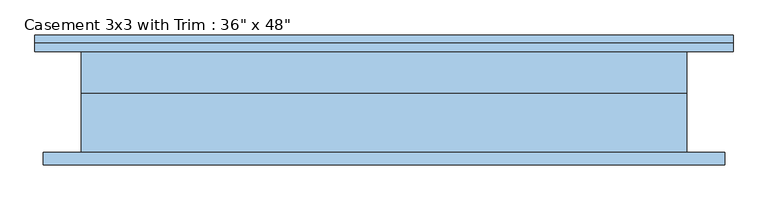
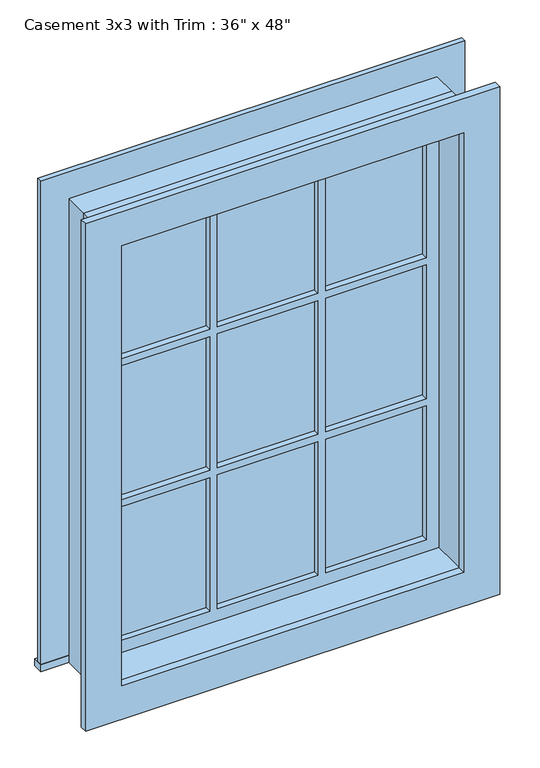
"""IFC4 building model written with IfcOpenShell, lengths in millimetres: window geometry."""

from ifc_helpers import new_model, si_unit, frame, origin, place, context, project, spatial, polyline, outline, extrude, source, transform, mapped, element, save


def window_5c190c7e(model_context):
    return source(origin(), model_context, "Body", "SweptSolid", [
        extrude(outline(polyline([(-527.05, 101.6), (527.05, 101.6), (527.05, 76.2), (-527.05, 76.2), (-527.05, 101.6)])), frame((0.0, 0.0, 914.4), z_axis=(0.0, 0.0, 1.0), x_axis=(1.0, 0.0, 0.0)), (0.0, 0.0, 1.0), 19.05),
        extrude(outline(polyline([(2114.55, -438.15), (2114.55, 438.15), (933.45, 438.15), (933.45, 527.05), (2203.45, 527.05), (2203.45, -527.05), (933.45, -527.05), (933.45, -438.15), (2114.55, -438.15)])), frame((0.0, 76.2, 0.0), z_axis=(0.0, 1.0, 0.0), x_axis=(0.0, 0.0, 1.0)), (0.0, 0.0, 1.0), 12.7),
        extrude(outline(polyline([(143.9333333, 41.275), (393.7, 41.275), (393.7, 28.575), (143.9333333, 28.575), (143.9333333, 41.275)])), frame((0.0, 0.0, 1718.7333333), z_axis=(0.0, 0.0, 1.0), x_axis=(1.0, 0.0, 0.0)), (0.0, 0.0, 1.0), 351.3666667),
        extrude(outline(polyline([(-124.8833333, 41.275), (124.8833333, 41.275), (124.8833333, 28.575), (-124.8833333, 28.575), (-124.8833333, 41.275)])), frame((0.0, 0.0, 1718.7333333), z_axis=(0.0, 0.0, 1.0), x_axis=(1.0, 0.0, 0.0)), (0.0, 0.0, 1.0), 351.3666667),
        extrude(outline(polyline([(-393.7, 41.275), (-143.9333333, 41.275), (-143.9333333, 28.575), (-393.7, 28.575), (-393.7, 41.275)])), frame((0.0, 0.0, 1718.7333333), z_axis=(0.0, 0.0, 1.0), x_axis=(1.0, 0.0, 0.0)), (0.0, 0.0, 1.0), 351.3666667),
        extrude(outline(polyline([(-393.7, 41.275), (-143.9333333, 41.275), (-143.9333333, 28.575), (-393.7, 28.575), (-393.7, 41.275)])), frame((0.0, 0.0, 1348.3166667), z_axis=(0.0, 0.0, 1.0), x_axis=(1.0, 0.0, 0.0)), (0.0, 0.0, 1.0), 351.3666667),
        extrude(outline(polyline([(-124.8833333, 41.275), (124.8833333, 41.275), (124.8833333, 28.575), (-124.8833333, 28.575), (-124.8833333, 41.275)])), frame((0.0, 0.0, 1348.3166667), z_axis=(0.0, 0.0, 1.0), x_axis=(1.0, 0.0, 0.0)), (0.0, 0.0, 1.0), 351.3666667),
        extrude(outline(polyline([(143.9333333, 41.275), (393.7, 41.275), (393.7, 28.575), (143.9333333, 28.575), (143.9333333, 41.275)])), frame((0.0, 0.0, 1348.3166667), z_axis=(0.0, 0.0, 1.0), x_axis=(1.0, 0.0, 0.0)), (0.0, 0.0, 1.0), 351.3666667),
        extrude(outline(polyline([(143.9333333, 41.275), (393.7, 41.275), (393.7, 28.575), (143.9333333, 28.575), (143.9333333, 41.275)])), frame((0.0, 0.0, 977.9), z_axis=(0.0, 0.0, 1.0), x_axis=(1.0, 0.0, 0.0)), (0.0, 0.0, 1.0), 351.3666667),
        extrude(outline(polyline([(-124.8833333, 41.275), (124.8833333, 41.275), (124.8833333, 28.575), (-124.8833333, 28.575), (-124.8833333, 41.275)])), frame((0.0, 0.0, 977.9), z_axis=(0.0, 0.0, 1.0), x_axis=(1.0, 0.0, 0.0)), (0.0, 0.0, 1.0), 351.3666667),
        extrude(outline(polyline([(-393.7, 41.275), (-143.9333333, 41.275), (-143.9333333, 28.575), (-393.7, 28.575), (-393.7, 41.275)])), frame((0.0, 0.0, 977.9), z_axis=(0.0, 0.0, 1.0), x_axis=(1.0, 0.0, 0.0)), (0.0, 0.0, 1.0), 351.3666667),
        extrude(outline(polyline([(2190.75, 514.35), (2190.75, -514.35), (857.25, -514.35), (857.25, 514.35), (2190.75, 514.35)]), holes=[polyline([(2101.85, 425.45), (946.15, 425.45), (946.15, -425.45), (2101.85, -425.45), (2101.85, 425.45)])]), frame((0.0, -95.25, 0.0), z_axis=(0.0, 1.0, 0.0), x_axis=(0.0, 0.0, 1.0)), (0.0, 0.0, 1.0), 19.05),
        extrude(outline(polyline([(2114.55, -438.15), (933.45, -438.15), (933.45, 438.15), (2114.55, 438.15), (2114.55, -438.15)]), holes=[polyline([(2070.1, -143.9333333), (1718.7333333, -143.9333333), (1718.7333333, -393.7), (2070.1, -393.7), (2070.1, -143.9333333)]), polyline([(1699.6833333, -143.9333333), (1348.3166667, -143.9333333), (1348.3166667, -393.7), (1699.6833333, -393.7), (1699.6833333, -143.9333333)]), polyline([(1329.2666667, -143.9333333), (977.9, -143.9333333), (977.9, -393.7), (1329.2666667, -393.7), (1329.2666667, -143.9333333)]), polyline([(2070.1, 124.8833333), (1718.7333333, 124.8833333), (1718.7333333, -124.8833333), (2070.1, -124.8833333), (2070.1, 124.8833333)]), polyline([(1699.6833333, 124.8833333), (1348.3166667, 124.8833333), (1348.3166667, -124.8833333), (1699.6833333, -124.8833333), (1699.6833333, 124.8833333)]), polyline([(1329.2666667, 124.8833333), (977.9, 124.8833333), (977.9, -124.8833333), (1329.2666667, -124.8833333), (1329.2666667, 124.8833333)]), polyline([(2070.1, 393.7), (1718.7333333, 393.7), (1718.7333333, 143.9333333), (2070.1, 143.9333333), (2070.1, 393.7)]), polyline([(1699.6833333, 393.7), (1348.3166667, 393.7), (1348.3166667, 143.9333333), (1699.6833333, 143.9333333), (1699.6833333, 393.7)]), polyline([(1329.2666667, 393.7), (977.9, 393.7), (977.9, 143.9333333), (1329.2666667, 143.9333333), (1329.2666667, 393.7)])]), frame((0.0, 12.7, 0.0), z_axis=(0.0, 1.0, 0.0), x_axis=(0.0, 0.0, 1.0)), (0.0, 0.0, 1.0), 44.45),
        extrude(outline(polyline([(2133.6, -457.2), (914.4, -457.2), (914.4, 457.2), (2133.6, 457.2), (2133.6, -457.2)]), holes=[polyline([(2101.85, -425.45), (2101.85, 425.45), (946.15, 425.45), (946.15, -425.45), (2101.85, -425.45)])]), frame((0.0, -76.2, 0.0), z_axis=(0.0, 1.0, 0.0), x_axis=(0.0, 0.0, 1.0)), (0.0, 0.0, 1.0), 88.9),
        extrude(outline(polyline([(2133.6, 457.2), (2133.6, -457.2), (914.4, -457.2), (914.4, 457.2), (2133.6, 457.2)]), holes=[polyline([(2114.55, 438.15), (933.45, 438.15), (933.45, -438.15), (2114.55, -438.15), (2114.55, 438.15)])]), frame((0.0, 12.7, 0.0), z_axis=(0.0, 1.0, 0.0), x_axis=(0.0, 0.0, 1.0)), (0.0, 0.0, 1.0), 63.5),
    ])


if __name__ == "__main__":
    model = new_model("IFC4")
    model_context = context("Model", 3, world=origin())
    ifc_project = project(units=[si_unit("LENGTHUNIT", "METRE", prefix="MILLI")], contexts=[model_context])
    site = spatial("IfcSite", under=ifc_project)
    building = spatial("IfcBuilding", under=site)
    placement = place(None, origin())
    window_shape = window_5c190c7e(model_context)
    element("IfcWindow", 1, ObjectType="Casement 3x3 with Trim : 36\" x 48\"", at=placement, inside=building, context=model_context, shape_type="MappedRepresentation", body=[
        mapped(window_shape, transform((0.0, 0.0, 0.0), x_axis=(1.0, 0.0, 0.0), y_axis=(0.0, 1.0, 0.0), z_axis=(0.0, 0.0, 1.0))),
    ])
    save(model, "model.ifc")

# Revit data of these elements
# Type "Casement 3x3 with Trim : 36\" x 48\""
#   Type Mark = "10"
#   Construction Type Id = "GSP4R"
#   Assembly Code = "B2020100"
#   Analytic Construction = "1/8 in Pilkington single glazing"
#   Visual Light Transmittance = 0.9
#   Solar Heat Gain Coefficient = 0.78
#   Heat Transfer Coefficient (U) = 0.6496 BTU/(h·ft²·°F)
#   Height = 4' - 0"
#   Default Sill Height = 3' - 0"
#   Trim Projection - Ext. = 0' - 0 1/2"
#   Trim Projection - Int. = 0' - 0 3/4"
#   Trim Width - Exterior = 0' - 3 1/2"
#   Trim Width - Interior = 0' - 3 1/2"
#   Width = 3' - 0"
#   Window Inset = 0' - 0 3/4"
#   Define Thermal Properties by = 1
#   Glass Pane Material = Glass
#   Sash Material = Sash
#   Trim Exterior Material = Trim
#   Trim Interior Material = Trim
#   Wall Closure = (empty or 0)
# Element 1 (IfcWindow, "Casement 3x3 with Trim : 36\" x 48\"")
#   Materials on its faces: "Sash", "Glass", "Trim"
# Materials
#   "Glass": class "Glass", colour RGB 0 128 192, transparency 0.75, Description = "Soda Lime Glass", Cost = 0
#   "Sash": class "Wood", colour RGB 224 178 126, transparency 0
#   "Trim": class "Wood", colour RGB 224 178 126, transparency 0
